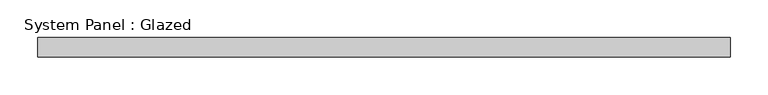
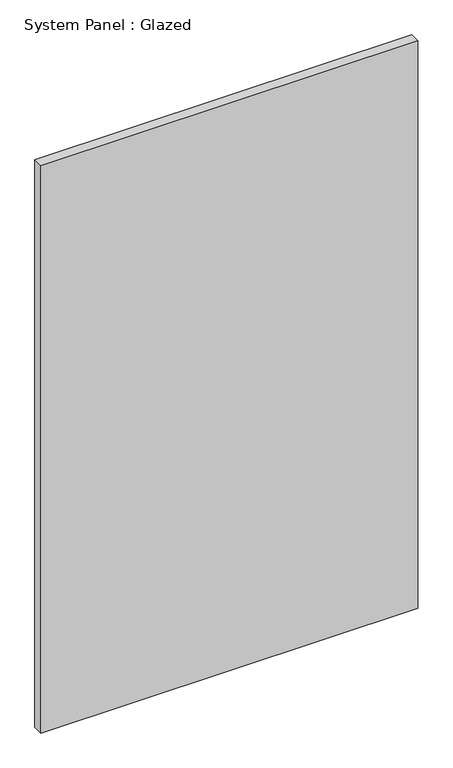
"""IFC4 building model written with IfcOpenShell, lengths in millimetres: plate geometry, System Panel : Glazed."""

from ifc_helpers import new_model, si_unit, origin, origin_with_axes, place, context, project, spatial, polyline, outline, extrude, source, transform, mapped, element, save


def system_panel_glazed_3397605a(model_context):
    return source(origin(), model_context, "Body", "SweptSolid", [
        extrude(outline(polyline([(457.2, 19.05), (-457.2, 19.05), (-457.2, 44.45), (457.2, 44.45), (457.2, 19.05)])), origin_with_axes(), (0.0, 0.0, 1.0), 1454.8539668),
    ])


if __name__ == "__main__":
    model = new_model("IFC4")
    model_context = context("Model", 3, world=origin())
    ifc_project = project(units=[si_unit("LENGTHUNIT", "METRE", prefix="MILLI")], contexts=[model_context])
    site = spatial("IfcSite", under=ifc_project)
    building = spatial("IfcBuilding", under=site)
    placement = place(None, origin())
    system_panel_glazed_shape = system_panel_glazed_3397605a(model_context)
    element("IfcPlate", 1, ObjectType="System Panel : Glazed", at=placement, inside=building, context=model_context, shape_type="MappedRepresentation", body=[
        mapped(system_panel_glazed_shape, transform((0.0, 0.0, 0.0), x_axis=(1.0, 0.0, 0.0), y_axis=(0.0, 1.0, 0.0), z_axis=(0.0, 0.0, 1.0))),
    ])
    save(model, "model.ifc")

# Revit data of these elements
# Type "System Panel : Glazed"
#   Construction Type Id = "GSP4R"
#   Analytic Construction = "1/8 in Pilkington single glazing"
#   Visual Light Transmittance = 0.9
#   Solar Heat Gain Coefficient = 0.86
#   Heat Transfer Coefficient (U) = 1.18115 BTU/(h·ft²·°F)
#   Define Thermal Properties by = 1
# Element 1 (IfcPlate, "System Panel : Glazed")
#   Materials on its faces: "Glass"
# Materials
#   "Glass": class "Glass", colour RGB 0 128 192, transparency 0.75, Description = "Soda Lime Glass", Cost = 0
